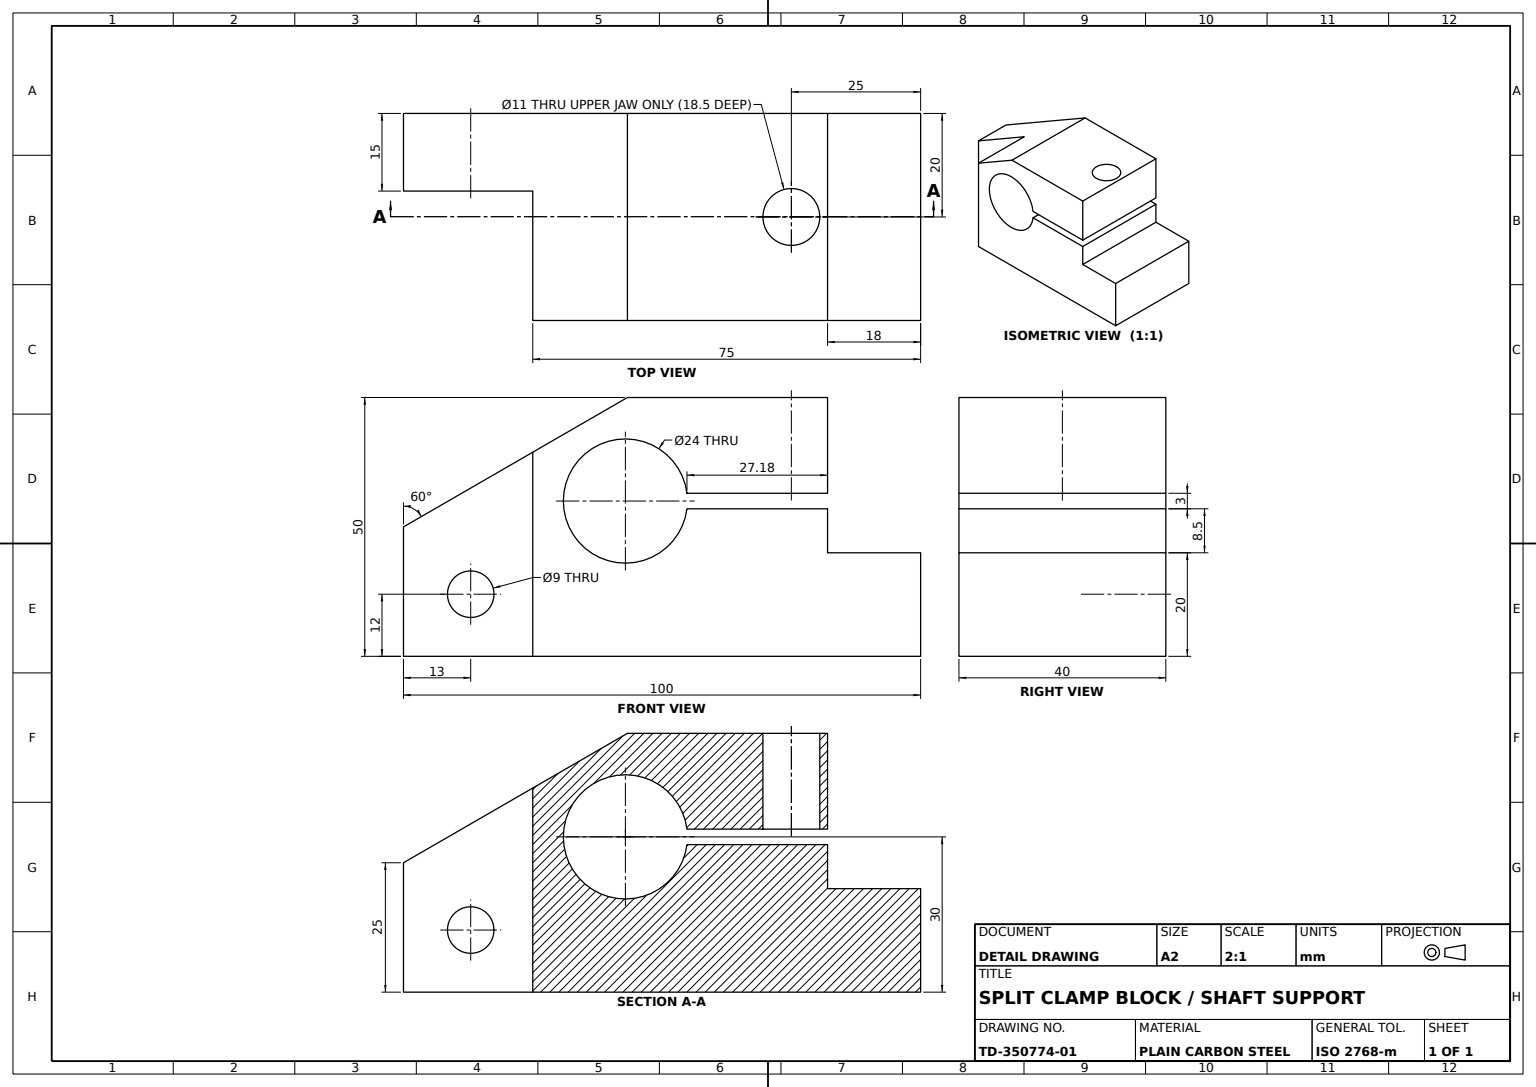
from build123d import *

# Parameters (mm, degrees)
BLOCK_BODY_DEPTH            = 40
CROSS_HOLE_SKETCH_R         = 4.5
CROSS_HOLE_DEPTH            = 87.622762369
RECTANGULAR_CUT_SKETCH_W    = 25
RECTANGULAR_CUT_SKETCH_H    = 25
RECTANGULAR_CUT_15X75_DEPTH = 87.622762369
TOP_CLAMP_HOLE_SKETCH_R     = 5.5
TOP_CLAMP_HOLE_DEPTH        = 18.5


with BuildPart() as part:
    # Block Profile Sketch → Block Body (new body)
    with BuildSketch(Plane.XY):
        with BuildLine():
            Line((-58.339548854, 25), (-58.339548854, 0))
            Line((-58.339548854, 0), (41.660451146, 0))
            Line((41.660451146, 0), (41.660451146, 20))
            Line((41.660451146, 20), (23.660451146, 20))
            Line((23.660451146, 20), (23.660451146, 28.5))
            Line((23.660451146, 28.5), (-3.52361978, 28.5))
            ThreePointArc((-3.52361978, 28.5), (-27.42950068, 30), (-3.52361978, 31.5))
            Line((-3.52361978, 31.5), (23.660451146, 31.5))
            Line((23.660451146, 31.5), (23.660451146, 50))
            Line((23.660451146, 50), (-15.038278665, 50))
            Line((-15.038278665, 50), (-58.339548854, 25))
        make_face()
    extrude(amount=BLOCK_BODY_DEPTH)

    # Cross Hole Sketch → Cross Hole (cut, through all)
    with BuildSketch(Plane.XY.offset(40)):
        with Locations((-45.339548854, 12)):
            Circle(CROSS_HOLE_SKETCH_R)
    extrude(amount=-CROSS_HOLE_DEPTH, mode=Mode.SUBTRACT)

    # Rectangular Cut Sketch → Rectangular Cut 15x75 (cut, through all)
    with BuildSketch(Plane.XZ):
        with Locations((-45.839548854, 27.5)):
            Rectangle(RECTANGULAR_CUT_SKETCH_W, RECTANGULAR_CUT_SKETCH_H)
    extrude(amount=-RECTANGULAR_CUT_15X75_DEPTH, mode=Mode.SUBTRACT)

    # Top Clamp Hole Sketch → Top Clamp Hole (cut)
    with BuildSketch(Plane(origin=(0, 50, 0), x_dir=(1, 0, 0), z_dir=(0, 1, 0))):
        with Locations(Location((16.660451146, -20, 0), (0, 0, 270))):
            Circle(TOP_CLAMP_HOLE_SKETCH_R)
    extrude(amount=-TOP_CLAMP_HOLE_DEPTH, mode=Mode.SUBTRACT)


solid = part.part
